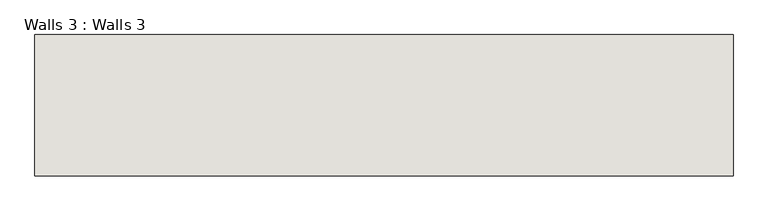
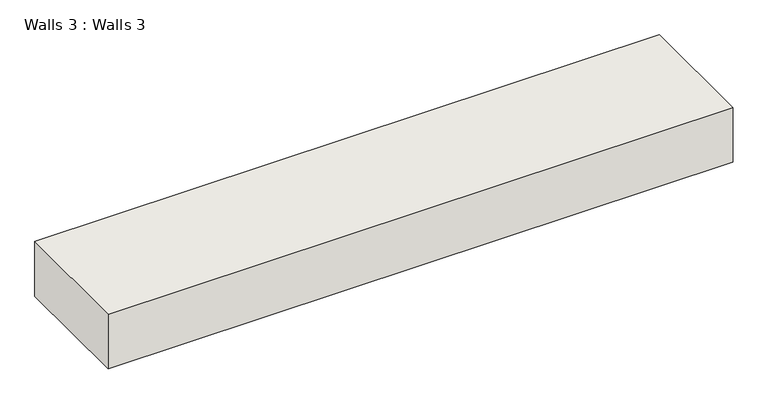
"""IFC4 building model written with IfcOpenShell, lengths in millimetres: wall geometry, Walls 3 : Walls 3."""

from ifc_helpers import new_model, si_unit, frame, origin, place, context, project, spatial, polyline, outline, extrude, source, transform, mapped, element, save


def walls_3_walls_3_551fdec1(model_context):
    return source(origin(), model_context, "Body", "SweptSolid", [
        extrude(outline(polyline([(6063.8250851, -3145.6291503), (-5213.7749149, -3145.6291503), (-5213.7749149, -860.9451257), (6063.8250851, -860.9451257), (6063.8250851, -3145.6291503)])), frame((0.0, 0.0, 10931.9442033), z_axis=(0.0, 0.0, 1.0), x_axis=(1.0, 0.0, 0.0)), (0.0, 0.0, 1.0), 1044.1583147),
    ])


if __name__ == "__main__":
    model = new_model("IFC4")
    model_context = context("Model", 3, world=origin())
    ifc_project = project(units=[si_unit("LENGTHUNIT", "METRE", prefix="MILLI")], contexts=[model_context])
    site = spatial("IfcSite", under=ifc_project)
    building = spatial("IfcBuilding", under=site)
    placement = place(None, origin())
    walls_3_walls_3_shape = walls_3_walls_3_551fdec1(model_context)
    element("IfcWall", 1, ObjectType="Walls 3 : Walls 3", at=placement, inside=building, context=model_context, shape_type="MappedRepresentation", body=[
        mapped(walls_3_walls_3_shape, transform((0.0, 0.0, 0.0), x_axis=(1.0, 0.0, 0.0), y_axis=(0.0, 1.0, 0.0), z_axis=(0.0, 0.0, 1.0))),
    ])
    save(model, "model.ifc")

# Revit data of these elements
# Element 1 (IfcWall, "Walls 3 : Walls 3")
#   Materials on its faces: "Default Wall"
# Materials
#   "Default Wall": colour RGB 128 128 128, transparency 0
